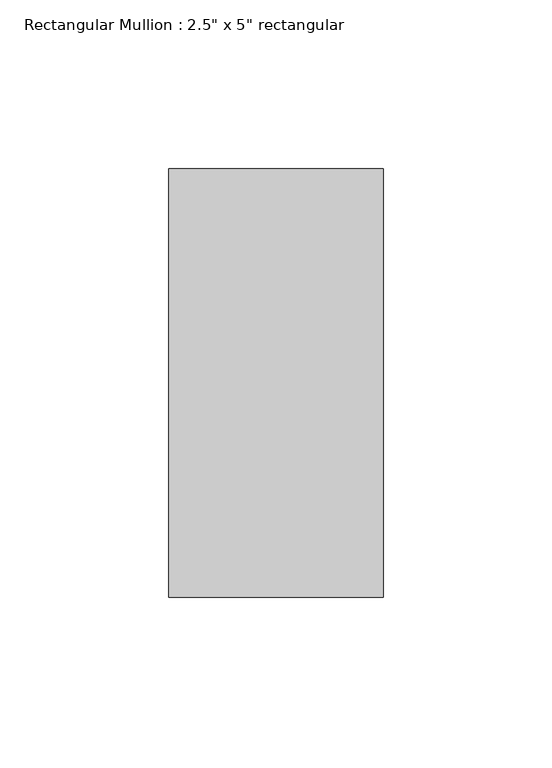
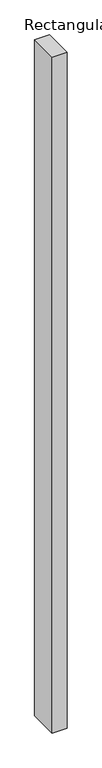
"""IFC4 building model written with IfcOpenShell, lengths in millimetres: member geometry."""

from ifc_helpers import new_model, si_unit, frame, origin, place, context, project, spatial, polyline, outline, extrude, source, transform, mapped, element, save


def member_cd64752f(model_context):
    return source(origin(), model_context, "Body", "SweptSolid", [
        extrude(outline(polyline([(0.0, 63.5), (0.0, -63.5), (-63.5, -63.5), (-63.5, 63.5), (0.0, 63.5)])), frame((0.0, 0.0, -3011.3632737), z_axis=(0.0, 0.0, 1.0), x_axis=(1.0, 0.0, 0.0)), (0.0, 0.0, 1.0), 3011.3632737),
    ])


if __name__ == "__main__":
    model = new_model("IFC4")
    model_context = context("Model", 3, world=origin())
    ifc_project = project(units=[si_unit("LENGTHUNIT", "METRE", prefix="MILLI")], contexts=[model_context])
    site = spatial("IfcSite", under=ifc_project)
    building = spatial("IfcBuilding", under=site)
    placement = place(None, origin())
    member_shape = member_cd64752f(model_context)
    element("IfcMember", 1, ObjectType="Rectangular Mullion : 2.5\" x 5\" rectangular", at=placement, inside=building, context=model_context, shape_type="MappedRepresentation", body=[
        mapped(member_shape, transform((0.0, 0.0, 0.0), x_axis=(1.0, 0.0, 0.0), y_axis=(0.0, 1.0, 0.0), z_axis=(0.0, 0.0, 1.0))),
    ])
    save(model, "model.ifc")

# Revit data of these elements
# Type "Rectangular Mullion : 2.5\" x 5\" rectangular"
#   built-in parameter 1007304 = 0.416667 (stored number, unit not read)
#   built-in parameter 1007301 = 0.104167 (stored number, unit not read)
#   built-in parameter 1007300 = 0.104167 (stored number, unit not read)
